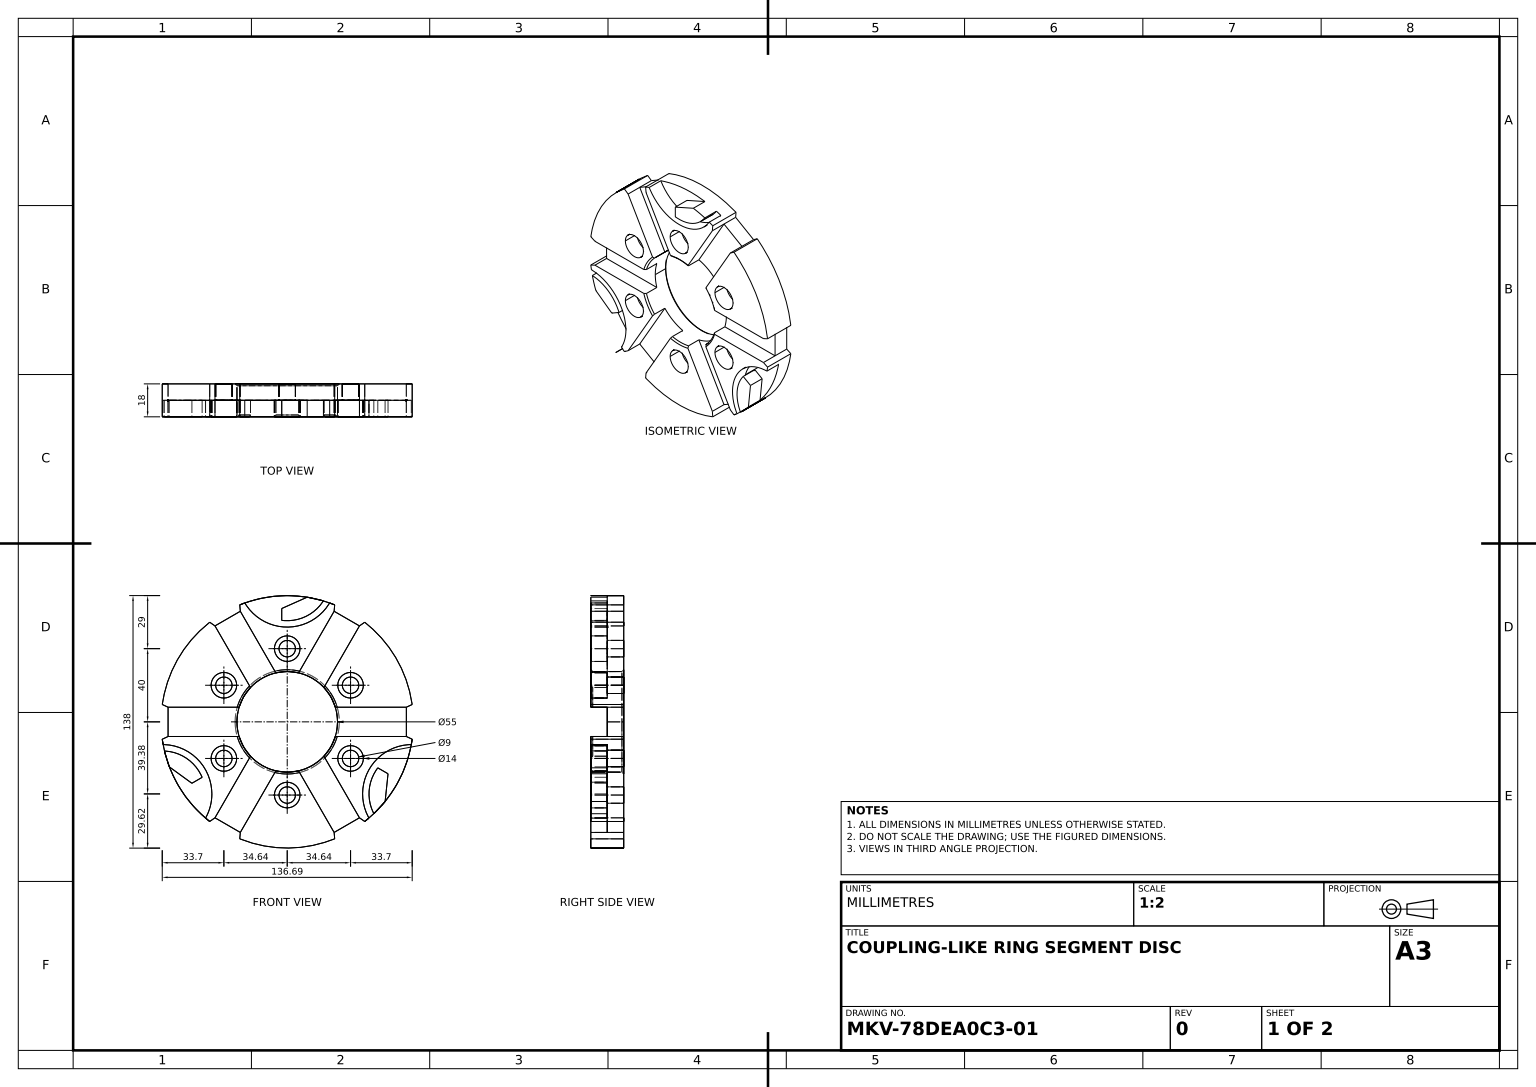
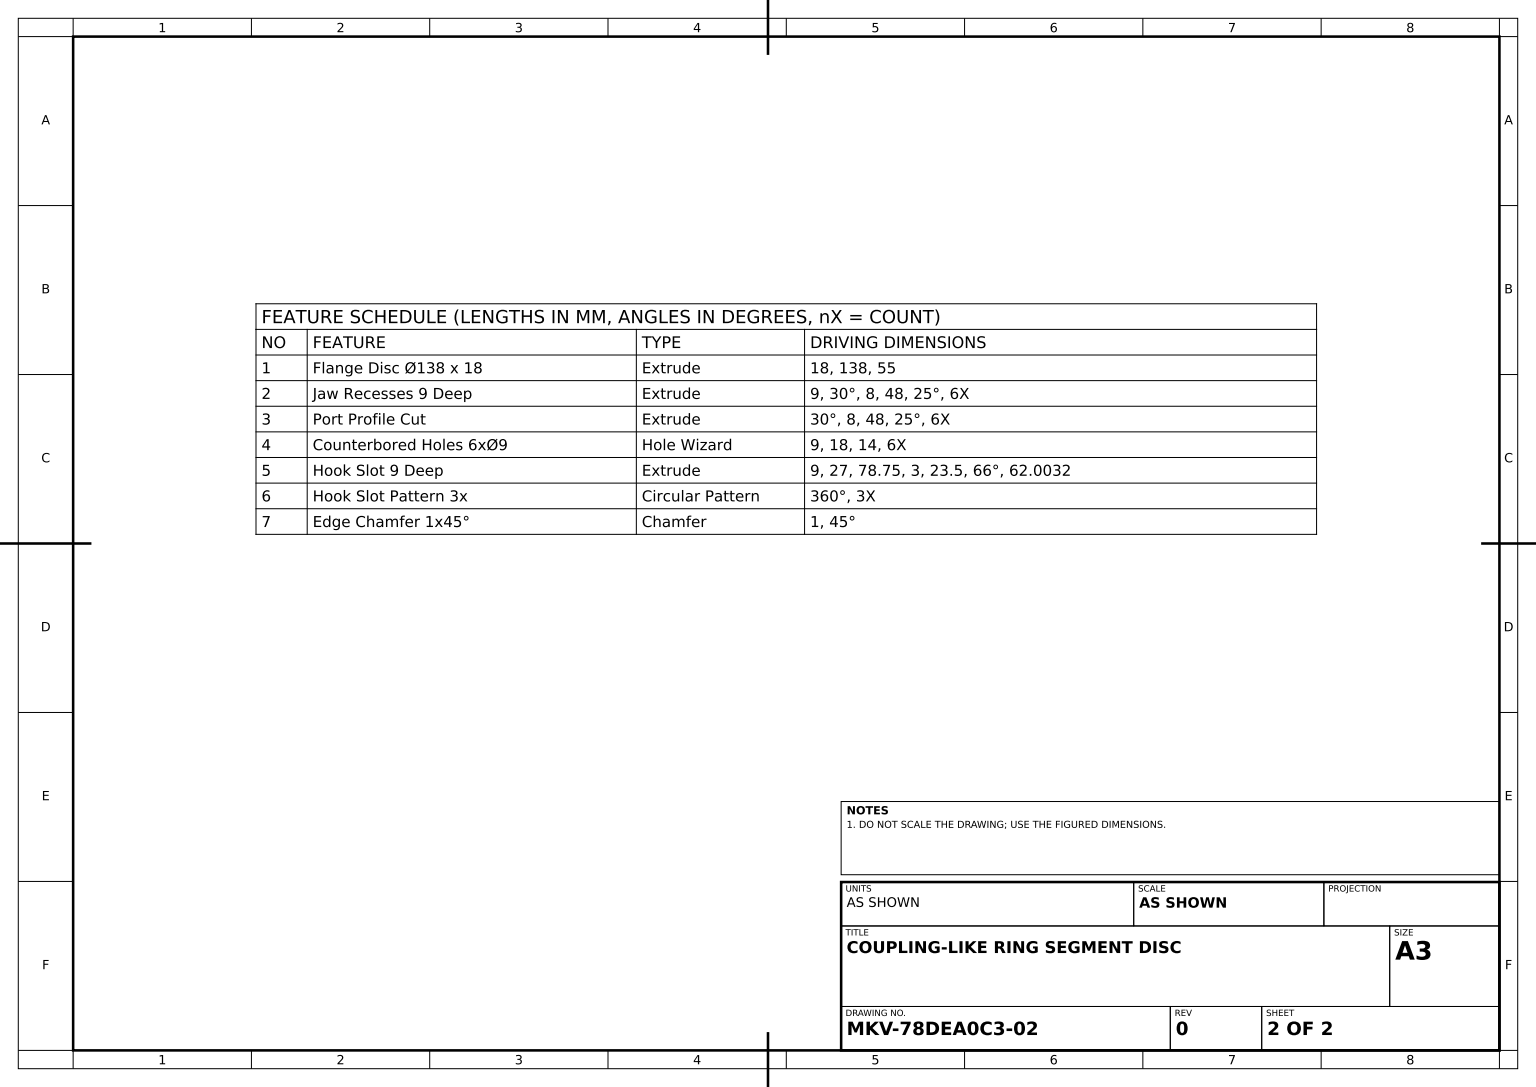
from build123d import *

# Parameters (mm, degrees)
FLANGE_DISC_SKETCH_R                = 69
FLANGE_DISC_SKETCH_R_2              = 27.5
FLANGE_DISC_138_X_18_DEPTH          = 18
JAW_START                           = -9
JAW_RECESSES_9_DEEP_DEPTH           = 9
PORT_PROFILE_CUT_DEPTH              = 100.227012451
COUNTERBORED_HOLES_6X_9_D           = 9
COUNTERBORED_HOLES_6X_9_CBORE_D     = 14
COUNTERBORED_HOLES_6X_9_CBORE_DEPTH = 9
HOOK_START                          = -9
HOOK_SLOT_9_DEEP_DEPTH              = 9
HOOK_SLOT_PATTERN_3X_COUNT          = 3
EDGE_CHAMFER_1X45_SIZE              = 1


with BuildPart() as part:
    # Flange Disc Sketch → Flange Disc _138 x 18 (new body)
    with BuildSketch(Plane.XY):
        Circle(FLANGE_DISC_SKETCH_R)
        Circle(FLANGE_DISC_SKETCH_R_2, mode=Mode.SUBTRACT)
    extrude(amount=FLANGE_DISC_138_X_18_DEPTH)

    # Jaw And Port Sketch → Jaw Recesses 9 Deep (cut)
    with BuildSketch(Plane.XY.offset(18).offset(JAW_START)):
        with BuildLine():
            ThreePointArc((-26.310644234, -8), (-27.5, 0), (-26.310644234, 8))
            Line((-26.310644234, 8), (-65.156055364, 8))
            Line((-65.156055364, 8), (-65.156055364, -8))
            Line((-65.156055364, -8), (-26.310644234, -8))
        make_face()
        with BuildLine():
            Line((-6.227118887, 26.785686296), (-25.649824452, 60.426799156))
            Line((-25.649824452, 60.426799156), (-39.506230912, 52.426799156))
            Line((-39.506230912, 52.426799156), (-20.083525347, 18.785686296))
            ThreePointArc((-20.083525347, 18.785686296), (-13.75, 23.815698604), (-6.227118887, 26.785686296))
        make_face()
        with BuildLine():
            Line((25.649824452, 60.426799156), (6.227118887, 26.785686296))
            ThreePointArc((6.227118887, 26.785686296), (13.75, 23.815698604), (20.083525347, 18.785686296))
            Line((20.083525347, 18.785686296), (39.506230912, 52.426799156))
            Line((39.506230912, 52.426799156), (25.649824452, 60.426799156))
        make_face()
        with BuildLine():
            Line((65.156055364, 8), (26.310644234, 8))
            ThreePointArc((26.310644234, 8), (27.201035977, 4.043963623), (27.5, 0))
            ThreePointArc((27.5, 0), (27.201035977, -4.043963623), (26.310644234, -8))
            Line((26.310644234, -8), (65.156055364, -8))
            Line((65.156055364, -8), (65.156055364, 8))
        make_face()
        with BuildLine():
            Line((39.506230912, -52.426799156), (20.083525347, -18.785686296))
            ThreePointArc((20.083525347, -18.785686296), (13.75, -23.815698604), (6.227118887, -26.785686296))
            Line((6.227118887, -26.785686296), (25.649824452, -60.426799156))
            Line((25.649824452, -60.426799156), (39.506230912, -52.426799156))
        make_face()
        with BuildLine():
            ThreePointArc((-6.227118887, -26.785686296), (-13.75, -23.815698604), (-20.083525347, -18.785686296))
            Line((-20.083525347, -18.785686296), (-39.506230912, -52.426799156))
            Line((-39.506230912, -52.426799156), (-25.649824452, -60.426799156))
            Line((-25.649824452, -60.426799156), (-6.227118887, -26.785686296))
        make_face()
    extrude(amount=JAW_RECESSES_9_DEEP_DEPTH, mode=Mode.SUBTRACT)

    # Sketch3_3 → Port Profile Cut (cut, through all)
    with BuildSketch(Plane.XY.offset(18)):
        with BuildLine():
            Line((-65.156055364, 8), (-68.344706261, 9.486892332))
            ThreePointArc((-68.344706261, 9.486892332), (-69, 0), (-68.344706261, -9.486892332))
            Line((-68.344706261, -9.486892332), (-65.156055364, -8))
            Line((-65.156055364, -8), (-65.156055364, 8))
        make_face()
        with BuildLine():
            Line((-39.506230912, -52.426799156), (-42.388242893, -54.44480567))
            ThreePointArc((-42.388242893, -54.44480567), (-34.5, -59.755752861), (-25.956463368, -63.931698002))
            Line((-25.956463368, -63.931698002), (-25.649824452, -60.426799156))
            Line((-25.649824452, -60.426799156), (-39.506230912, -52.426799156))
        make_face()
        with BuildLine():
            ThreePointArc((25.956463368, -63.931698002), (34.5, -59.755752861), (42.388242893, -54.44480567))
            Line((42.388242893, -54.44480567), (39.506230912, -52.426799156))
            Line((39.506230912, -52.426799156), (25.649824452, -60.426799156))
            Line((25.649824452, -60.426799156), (25.956463368, -63.931698002))
        make_face()
        with BuildLine():
            ThreePointArc((69, 0), (68.835981623, 4.754748574), (68.344706261, 9.486892332))
            Line((68.344706261, 9.486892332), (65.156055364, 8))
            Line((65.156055364, 8), (65.156055364, -8))
            Line((65.156055364, -8), (68.344706261, -9.486892332))
            ThreePointArc((68.344706261, -9.486892332), (68.835981623, -4.754748574), (69, 0))
        make_face()
        with BuildLine():
            ThreePointArc((42.388242893, 54.44480567), (34.5, 59.755752861), (25.956463368, 63.931698002))
            Line((25.956463368, 63.931698002), (25.649824452, 60.426799156))
            Line((25.649824452, 60.426799156), (39.506230912, 52.426799156))
            Line((39.506230912, 52.426799156), (42.388242893, 54.44480567))
        make_face()
        with BuildLine():
            Line((-39.506230912, 52.426799156), (-25.649824452, 60.426799156))
            Line((-25.649824452, 60.426799156), (-25.956463368, 63.931698002))
            ThreePointArc((-25.956463368, 63.931698002), (-34.5, 59.755752861), (-42.388242893, 54.44480567))
            Line((-42.388242893, 54.44480567), (-39.506230912, 52.426799156))
        make_face()
    extrude(amount=-PORT_PROFILE_CUT_DEPTH, mode=Mode.SUBTRACT)

    # Counterbored Holes 6x_9 (through all)
    with Locations(Plane.XY.offset(18)):
        with Locations((0, 40), (34.641016151, 20), (34.641016151, -20), (0, -40), (-34.641016151, -20), (-34.641016151, 20)):
            CounterBoreHole(COUNTERBORED_HOLES_6X_9_D / 2, COUNTERBORED_HOLES_6X_9_CBORE_D / 2, COUNTERBORED_HOLES_6X_9_CBORE_DEPTH)

    # Hook Slot Sketch → Hook Slot 9 Deep (cut)
    with BuildSketch(Plane.XY.offset(18).offset(HOOK_START)):
        with BuildLine():
            ThreePointArc((-67.143353435, -15.898744905), (-54.735535714, -20.114375634), (-46.514419424, -30.319214191))
            Line((-46.514419424, -30.319214191), (-52.133433448, -33.56335345))
            Line((-52.133433448, -33.56335345), (-64.464030022, -24.604650643))
            ThreePointArc((-64.464030022, -24.604650643), (-56.328274682, -39.851291966), (-44.65912882, -52.598119862))
            ThreePointArc((-44.65912882, -52.598119862), (-44.816814646, -25.875), (-67.880872402, -12.376880138))
            ThreePointArc((-67.880872402, -12.376880138), (-67.535074395, -14.142620919), (-67.143353435, -15.898744905))
        make_face()
    hook_slot_9_deep = extrude(amount=HOOK_SLOT_9_DEEP_DEPTH, mode=Mode.SUBTRACT)

    # Hook Slot Pattern 3x: Hook Slot 9 Deep ×3 about axis
    hook_slot_pattern_3x_axis = Axis((0, 0, 0), (0, 0, 1))
    for i in range(1, HOOK_SLOT_PATTERN_3X_COUNT):
        add(hook_slot_9_deep.rotate(hook_slot_pattern_3x_axis, i * 360 / HOOK_SLOT_PATTERN_3X_COUNT), mode=Mode.SUBTRACT)

    # Edge Chamfer 1x45
    edge_chamfer_1x45_edges = [part.edges().sort_by_distance(p)[0] for p in [
        (0, 27.5, 18),
        (-23.815698604, 13.75, 18),
        (-23.815698604, -13.75, 18),
        (0, -27.5, 18),
        (23.815698604, -13.75, 18),
        (-27.5, 0, 0),
        (23.815698604, 13.75, 18),
    ]]
    chamfer(edge_chamfer_1x45_edges, length=EDGE_CHAMFER_1X45_SIZE)


solid = part.part
